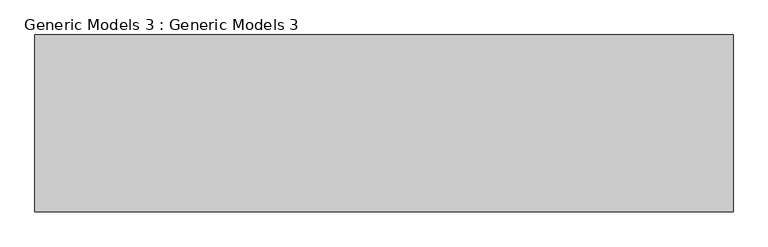
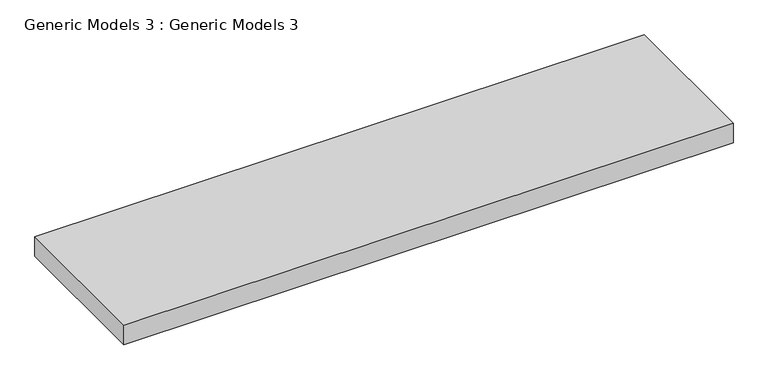
"""IFC4 building model written with IfcOpenShell, lengths in millimetres: proxy geometry, Generic Models 3 : Generic Models 3."""

from ifc_helpers import new_model, si_unit, origin, place, context, project, spatial, faceted_brep, source, transform, mapped, element, save


def generic_models_3_generic_models_3_5e2efcd9(model_context):
    return source(origin(), model_context, "Body", "Brep", [
        faceted_brep([(-4578.2831929, -11795.1399126, 3048.0), (-10534.5831929, -11795.1399126, 3048.0), (-10534.5831929, -11795.1399126, 2845.4571484), (-4578.2831929, -11795.1399126, 2845.4571484), (-4578.2831929, -10286.4592534, 3048.0), (-4578.2831929, -10286.4592534, 2845.4571484), (-4590.9831929, -10286.4592534, 2845.4571484), (-4971.9831929, -10286.4592534, 2845.4571484), (-10178.9831929, -10286.4592534, 2845.4571484), (-10534.5831929, -10286.4592534, 2845.4571484), (-10534.5831929, -10286.4592534, 3048.0), (-4971.9831929, -10286.4592534, 3048.0), (-4590.9831929, -10286.4592534, 3048.0), (-10534.5831929, -11734.2592534, 2845.4571484)], [[[0, 1, 2, 3]], [[4, 5, 6, 7, 8, 9, 10, 11, 12]], [[1, 0, 4, 12, 11, 10]], [[2, 1, 10, 9, 13]], [[3, 2, 13, 9, 8, 7, 6, 5]], [[0, 3, 5, 4]]]),
    ])


if __name__ == "__main__":
    model = new_model("IFC4")
    model_context = context("Model", 3, world=origin())
    ifc_project = project(units=[si_unit("LENGTHUNIT", "METRE", prefix="MILLI")], contexts=[model_context])
    site = spatial("IfcSite", under=ifc_project)
    building = spatial("IfcBuilding", under=site)
    placement = place(None, origin())
    generic_models_3_generic_models_3_shape = generic_models_3_generic_models_3_5e2efcd9(model_context)
    element("IfcBuildingElementProxy", 1, Name="Generic Models 3 : Generic Models 3", ObjectType="Generic Models 3 : Generic Models 3", at=placement, inside=building, context=model_context, shape_type="MappedRepresentation", body=[
        mapped(generic_models_3_generic_models_3_shape, transform((0.0, 0.0, 0.0), x_axis=(1.0, 0.0, 0.0), y_axis=(0.0, 1.0, 0.0), z_axis=(0.0, 0.0, 1.0))),
    ])
    save(model, "model.ifc")
